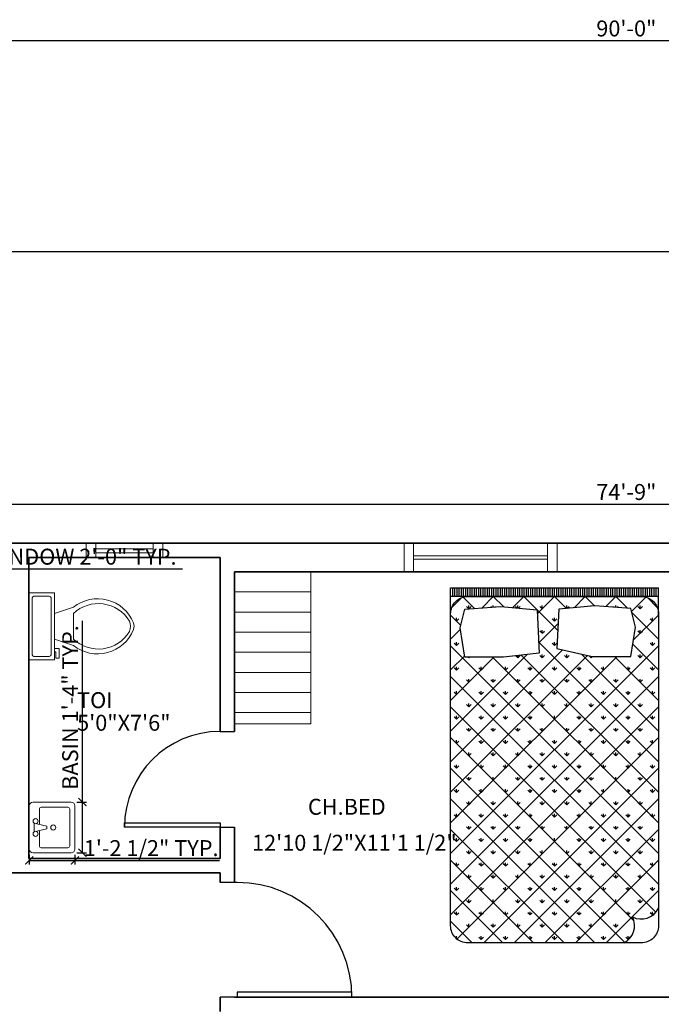
# Model space of a CAD drawing. Units: inches. Extents: x 3283068 to 3284536, y 3240756 to 3241803.
# Tile 15 of 19: x 3283598 to 3283799, y 3241494 to 3241803. Entities that reach past the tile are written whole.
import ezdxf

# ---------------------------------------------------------------- set-up
doc = ezdxf.new("R2010")
doc.units = ezdxf.units.IN
for name, color, linetype, lineweight in [('A-ANNO-DIMS', 2, 'Continuous', 18), ('A-AREA-IDEN', 7, 'Continuous', 18), ('A-FLOR-FIXT', 9, 'Continuous', 18), ('C-PROP', 7, 'Continuous', 25), ('door', 140, 'Continuous', 25), ('furniture', 40, 'Continuous', 18), ('wall', 20, 'Continuous', 35), ('wardrobe', 180, 'Continuous', 18), ('window', 100, 'Continuous', 18)]:
    doc.layers.add(name, color=color, linetype=linetype, lineweight=lineweight)
doc.layers.add('NOI THAT', color=42, linetype='Continuous')
doc.styles.get("Standard").update_dxf_attribs({"font": 'arial.ttf'})
doc.dimstyles.new('ISO-25', dxfattribs={"dimtxt": 5, "dimasz": 2.5, "dimexe": 1.25, "dimexo": 0.625, "dimtad": 1, "dimlunit": 4, "dimtxsty": 'Standard', "dimblk": 'ARCHTICK', "dimcen": 2.5, "dimadec": 0, "dimazin": 0, "dimtfac": 1, "dimtmove": 0, "dimatfit": 3, "dimfxl": 1, "dimarcsym": 0})

# ---------------------------------------------------------------- blocks, each defined once
blk = doc.blocks.new('*U6')
for p, q in [((0, 0), (0, -6)), ((-40, 0), (-40, -6))]:
    blk.add_line(p, q)
blk.add_lwpolyline([(0, 0), (0, 40), (-1.75, 40), (-1.75, 0)], close=True)
blk.add_arc((0, 0), 40, 90, 180)
blk = doc.blocks.new('*U5')
for p, q in [((-40, 0), (-40, 6)), ((0, 0), (0, 6))]:
    blk.add_line(p, q)
blk.add_lwpolyline([(0, 0), (0, -40), (-1.75, -40), (-1.75, 0)], close=True)
blk.add_arc((0, 0), 40, 180, 270)
blk = doc.blocks.new('*X15')
at = {"color": 0}
for p, q in [((-424.3, 0), (-424.3, 0)), ((-424.3, 0), (-424.3, 0)), ((-141.4, 0), (-141.4, 0)), ((-495, -70.6), (-495, -52)), ((-353.6, -60.2), (-353.6, -52)), ((-282.8, 0), (-282.8, 0)), ((-282.8, 0), (-282.8, 0)), ((-212.1, -65.8), (-212.1, -52)), ((-70.7, -70.7), (-70.7, -52)), ((70.7, -68.1), (70.7, -52)), ((212.1, -55), (212.1, -52)), ((282.8, 0), (282.8, 0)), ((353.6, -61.9), (353.6, -52)), ((424.3, 0), (424.3, 0)), ((495, -70.7), (495, -52)), ((-495.1, -70.6), (-508.2, -57.5)), ((-494.9, -70.6), (-481.7, -57.5)), ((-363.4, -60.9), (-366.8, -57.5)), ((-342.2, -59.3), (-340.3, -57.5)), ((-217.5, -65.3), (-225.4, -57.5)), ((-207.7, -66.2), (-198.9, -57.5)), ((-70.7, -70.7), (-84, -57.5)), ((-70.7, -70.7), (-57.5, -57.5)), ((68.3, -68.3), (57.5, -57.5)), ((73.6, -67.8), (84, -57.5)), ((344.1, -61.2), (340.3, -57.5)), ((361.7, -62.5), (366.8, -57.5)), ((495, -70.7), (481.7, -57.5)), ((495, -70.7), (508.2, -57.5)), ((-565.7, -141.4), (-578.9, -128.2)), ((-565.7, -141.4), (-565.7, -122.7)), ((-565.7, -141.4), (-552.4, -128.2)), ((0, -141.4), (-13.3, -128.2)), ((0, -141.4), (0, -122.7)), ((0, -141.4), (13.3, -128.2)), ((565.7, -141.4), (552.4, -128.2)), ((565.7, -141.4), (565.7, -122.7)), ((565.7, -141.4), (578.9, -128.2)), ((-70.7, -212.1), (-84, -198.9)), ((-70.7, -212.1), (-70.7, -193.4)), ((-70.7, -212.1), (-57.5, -198.9)), ((495, -212.1), (481.7, -198.9)), ((495, -212.1), (495, -193.4)), ((495, -212.1), (508.2, -198.9)), ((-565.7, -282.8), (-578.9, -269.6)), ((-565.7, -282.8), (-565.7, -264.1)), ((-565.7, -282.8), (-552.4, -269.6)), ((0, -282.8), (-13.3, -269.6)), ((0, -282.8), (0, -264.1)), ((0, -282.8), (13.3, -269.6)), ((565.7, -282.8), (552.4, -269.6)), ((565.7, -282.8), (565.7, -264.1)), ((565.7, -282.8), (578.9, -269.6)), ((-212.1, -353.6), (-212.1, -340.3)), ((-212.1, -353.6), (-198.9, -340.3)), ((-70.7, -353.6), (-84, -340.3)), ((-70.7, -353.6), (-70.7, -334.8)), ((-70.7, -353.6), (-57.5, -340.3)), ((70.7, -353.6), (57.5, -340.3)), ((70.7, -353.6), (70.7, -334.8)), ((70.7, -353.6), (84, -340.3)), ((495, -353.6), (481.7, -340.3)), ((495, -353.6), (495, -334.8)), ((495, -353.6), (508.2, -340.3)), ((-495, -353.6), (-499, -349.5)), ((-495, -353.6), (-495, -349.5)), ((-495, -353.6), (-491, -349.5)), ((-353.6, -353.6), (-357.6, -349.5)), ((-353.6, -353.6), (-353.6, -349.5)), ((-353.6, -353.6), (-349.5, -349.5)), ((-212.1, -353.6), (-224, -341.7)), ((212.1, -353.6), (200.4, -341.8)), ((212.1, -353.6), (212.1, -344.4)), ((212.1, -353.6), (220, -345.7)), ((353.6, -353.6), (345.7, -345.7)), ((353.6, -353.6), (353.6, -345.7)), ((353.6, -353.6), (361.4, -345.7)), ((-565.7, -424.3), (-578.9, -411)), ((-565.7, -424.3), (-565.7, -405.5)), ((-565.7, -424.3), (-552.4, -411)), ((-424.3, -424.3), (-437.5, -411)), ((-424.3, -424.3), (-424.3, -405.5)), ((-424.3, -424.3), (-411, -411)), ((-282.8, -424.3), (-296.1, -411)), ((-282.8, -424.3), (-282.8, -405.5)), ((-282.8, -424.3), (-269.6, -411)), ((-141.4, -424.3), (-154.7, -411)), ((-141.4, -424.3), (-141.4, -405.5)), ((-141.4, -424.3), (-128.2, -411)), ((0, -424.3), (-13.3, -411)), ((0, -424.3), (0, -405.5)), ((0, -424.3), (13.3, -411)), ((141.4, -424.3), (128.2, -411)), ((141.4, -424.3), (141.4, -405.5)), ((141.4, -424.3), (154.7, -411)), ((282.8, -424.3), (269.6, -411)), ((282.8, -424.3), (282.8, -405.5)), ((282.8, -424.3), (296.1, -411)), ((424.3, -424.3), (411, -411)), ((424.3, -424.3), (424.3, -405.5)), ((424.3, -424.3), (437.5, -411)), ((565.7, -424.3), (552.4, -411)), ((565.7, -424.3), (565.7, -405.5)), ((565.7, -424.3), (578.9, -411)), ((-495, -495), (-508.2, -481.7)), ((-495, -495), (-495, -476.2)), ((-495, -495), (-481.7, -481.7)), ((-353.6, -495), (-366.8, -481.7)), ((-353.6, -495), (-353.6, -476.2)), ((-353.6, -495), (-340.3, -481.7)), ((-212.1, -495), (-225.4, -481.7)), ((-212.1, -495), (-212.1, -476.2)), ((-212.1, -495), (-198.9, -481.7)), ((-70.7, -495), (-84, -481.7)), ((-70.7, -495), (-70.7, -476.2)), ((-70.7, -495), (-57.5, -481.7)), ((70.7, -495), (57.5, -481.7)), ((70.7, -495), (70.7, -476.2)), ((70.7, -495), (84, -481.7)), ((212.1, -495), (198.9, -481.7)), ((212.1, -495), (212.1, -476.2)), ((212.1, -495), (225.4, -481.7)), ((353.6, -495), (340.3, -481.7)), ((353.6, -495), (353.6, -476.2)), ((353.6, -495), (366.8, -481.7)), ((495, -495), (481.7, -481.7)), ((495, -495), (495, -476.2)), ((495, -495), (508.2, -481.7)), ((-565.7, -565.7), (-578.9, -552.4)), ((-565.7, -565.7), (-565.7, -546.9)), ((-565.7, -565.7), (-552.4, -552.4)), ((-424.3, -565.7), (-437.5, -552.4)), ((-424.3, -565.7), (-424.3, -546.9)), ((-424.3, -565.7), (-411, -552.4)), ((-282.8, -565.7), (-296.1, -552.4)), ((-282.8, -565.7), (-282.8, -546.9)), ((-282.8, -565.7), (-269.6, -552.4)), ((-141.4, -565.7), (-154.7, -552.4)), ((-141.4, -565.7), (-141.4, -546.9)), ((-141.4, -565.7), (-128.2, -552.4)), ((0, -565.7), (-13.3, -552.4)), ((0, -565.7), (0, -546.9)), ((0, -565.7), (13.3, -552.4)), ((141.4, -565.7), (128.2, -552.4)), ((141.4, -565.7), (141.4, -546.9)), ((141.4, -565.7), (154.7, -552.4)), ((282.8, -565.7), (269.6, -552.4)), ((282.8, -565.7), (282.8, -546.9)), ((282.8, -565.7), (296.1, -552.4)), ((424.3, -565.7), (411, -552.4)), ((424.3, -565.7), (424.3, -546.9)), ((424.3, -565.7), (437.5, -552.4)), ((565.7, -565.7), (552.4, -552.4)), ((565.7, -565.7), (565.7, -546.9)), ((565.7, -565.7), (578.9, -552.4)), ((-495, -636.4), (-508.2, -623.1)), ((-495, -636.4), (-495, -617.6)), ((-495, -636.4), (-481.7, -623.1)), ((-353.6, -636.4), (-366.8, -623.1)), ((-353.6, -636.4), (-353.6, -617.6)), ((-353.6, -636.4), (-340.3, -623.1)), ((-212.1, -636.4), (-225.4, -623.1)), ((-212.1, -636.4), (-212.1, -617.6)), ((-212.1, -636.4), (-198.9, -623.1)), ((-70.7, -636.4), (-84, -623.1)), ((-70.7, -636.4), (-70.7, -617.6)), ((-70.7, -636.4), (-57.5, -623.1)), ((70.7, -636.4), (57.5, -623.1)), ((70.7, -636.4), (70.7, -617.6)), ((70.7, -636.4), (84, -623.1)), ((212.1, -636.4), (198.9, -623.1)), ((212.1, -636.4), (212.1, -617.6)), ((212.1, -636.4), (225.4, -623.1)), ((353.6, -636.4), (340.3, -623.1)), ((353.6, -636.4), (353.6, -617.6)), ((353.6, -636.4), (366.8, -623.1)), ((495, -636.4), (481.7, -623.1)), ((495, -636.4), (495, -617.6)), ((495, -636.4), (508.2, -623.1)), ((-565.7, -707.1), (-578.9, -693.8)), ((-565.7, -707.1), (-565.7, -688.4)), ((-565.7, -707.1), (-552.4, -693.8)), ((-424.3, -707.1), (-437.5, -693.8)), ((-424.3, -707.1), (-424.3, -688.4)), ((-424.3, -707.1), (-411, -693.8)), ((-282.8, -707.1), (-296.1, -693.8)), ((-282.8, -707.1), (-282.8, -688.4)), ((-282.8, -707.1), (-269.6, -693.8)), ((-141.4, -707.1), (-154.7, -693.8)), ((-141.4, -707.1), (-141.4, -688.4)), ((-141.4, -707.1), (-128.2, -693.8)), ((0, -707.1), (-13.3, -693.8)), ((0, -707.1), (0, -688.4)), ((0, -707.1), (13.3, -693.8)), ((141.4, -707.1), (128.2, -693.8)), ((141.4, -707.1), (141.4, -688.4)), ((141.4, -707.1), (154.7, -693.8)), ((282.8, -707.1), (269.6, -693.8)), ((282.8, -707.1), (282.8, -688.4)), ((282.8, -707.1), (296.1, -693.8)), ((424.3, -707.1), (411, -693.8)), ((424.3, -707.1), (424.3, -688.4)), ((424.3, -707.1), (437.5, -693.8)), ((565.7, -707.1), (552.4, -693.8)), ((565.7, -707.1), (565.7, -688.4)), ((565.7, -707.1), (578.9, -693.8)), ((-495, -777.8), (-508.2, -764.6)), ((-495, -777.8), (-495, -759.1)), ((-495, -777.8), (-481.7, -764.6)), ((-353.6, -777.8), (-366.8, -764.6)), ((-353.6, -777.8), (-353.6, -759.1)), ((-353.6, -777.8), (-340.3, -764.6)), ((-212.1, -777.8), (-225.4, -764.6)), ((-212.1, -777.8), (-212.1, -759.1)), ((-212.1, -777.8), (-198.9, -764.6)), ((-70.7, -777.8), (-84, -764.6)), ((-70.7, -777.8), (-70.7, -759.1)), ((-70.7, -777.8), (-57.5, -764.6)), ((70.7, -777.8), (57.5, -764.6)), ((70.7, -777.8), (70.7, -759.1)), ((70.7, -777.8), (84, -764.6)), ((212.1, -777.8), (198.9, -764.6)), ((212.1, -777.8), (212.1, -759.1)), ((212.1, -777.8), (225.4, -764.6)), ((353.6, -777.8), (340.3, -764.6)), ((353.6, -777.8), (353.6, -759.1)), ((353.6, -777.8), (366.8, -764.6)), ((495, -777.8), (481.7, -764.6)), ((495, -777.8), (495, -759.1)), ((495, -777.8), (508.2, -764.6)), ((-565.7, -848.5), (-578.9, -835.3)), ((-565.7, -848.5), (-565.7, -829.8)), ((-565.7, -848.5), (-552.4, -835.3)), ((-424.3, -848.5), (-437.5, -835.3)), ((-424.3, -848.5), (-424.3, -829.8)), ((-424.3, -848.5), (-411, -835.3)), ((-282.8, -848.5), (-296.1, -835.3)), ((-282.8, -848.5), (-282.8, -829.8)), ((-282.8, -848.5), (-269.6, -835.3)), ((-141.4, -848.5), (-154.7, -835.3)), ((-141.4, -848.5), (-141.4, -829.8)), ((-141.4, -848.5), (-128.2, -835.3)), ((0, -848.5), (-13.3, -835.3)), ((0, -848.5), (0, -829.8)), ((0, -848.5), (13.3, -835.3)), ((141.4, -848.5), (128.2, -835.3)), ((141.4, -848.5), (141.4, -829.8)), ((141.4, -848.5), (154.7, -835.3)), ((282.8, -848.5), (269.6, -835.3)), ((282.8, -848.5), (282.8, -829.8)), ((282.8, -848.5), (296.1, -835.3)), ((424.3, -848.5), (411, -835.3)), ((424.3, -848.5), (424.3, -829.8)), ((424.3, -848.5), (437.5, -835.3)), ((565.7, -848.5), (552.4, -835.3)), ((565.7, -848.5), (565.7, -829.8)), ((565.7, -848.5), (578.9, -835.3)), ((-495, -919.2), (-508.2, -906)), ((-495, -919.2), (-495, -900.5)), ((-495, -919.2), (-481.7, -906)), ((-353.6, -919.2), (-366.8, -906)), ((-353.6, -919.2), (-353.6, -900.5)), ((-353.6, -919.2), (-340.3, -906)), ((-212.1, -919.2), (-225.4, -906)), ((-212.1, -919.2), (-212.1, -900.5)), ((-212.1, -919.2), (-198.9, -906)), ((-70.7, -919.2), (-84, -906)), ((-70.7, -919.2), (-70.7, -900.5)), ((-70.7, -919.2), (-57.5, -906)), ((70.7, -919.2), (57.5, -906)), ((70.7, -919.2), (70.7, -900.5)), ((70.7, -919.2), (84, -906)), ((212.1, -919.2), (198.9, -906)), ((212.1, -919.2), (212.1, -900.5)), ((212.1, -919.2), (225.4, -906)), ((353.6, -919.2), (340.3, -906)), ((353.6, -919.2), (353.6, -900.5)), ((353.6, -919.2), (366.8, -906)), ((495, -919.2), (481.7, -906)), ((495, -919.2), (495, -900.5)), ((495, -919.2), (508.2, -906)), ((-565.7, -989.9), (-578.9, -976.7)), ((-565.7, -989.9), (-565.7, -971.2)), ((-565.7, -989.9), (-552.4, -976.7)), ((-424.3, -989.9), (-437.5, -976.7)), ((-424.3, -989.9), (-424.3, -971.2)), ((-424.3, -989.9), (-411, -976.7)), ((-282.8, -989.9), (-296.1, -976.7)), ((-282.8, -989.9), (-282.8, -971.2)), ((-282.8, -989.9), (-269.6, -976.7)), ((-141.4, -989.9), (-154.7, -976.7)), ((-141.4, -989.9), (-141.4, -971.2)), ((-141.4, -989.9), (-128.2, -976.7)), ((0, -989.9), (-13.3, -976.7)), ((0, -989.9), (0, -971.2)), ((0, -989.9), (13.3, -976.7)), ((141.4, -989.9), (128.2, -976.7)), ((141.4, -989.9), (141.4, -971.2)), ((141.4, -989.9), (154.7, -976.7)), ((282.8, -989.9), (269.6, -976.7)), ((282.8, -989.9), (282.8, -971.2)), ((282.8, -989.9), (296.1, -976.7)), ((424.3, -989.9), (411, -976.7)), ((424.3, -989.9), (424.3, -971.2)), ((424.3, -989.9), (437.5, -976.7)), ((565.7, -989.9), (552.4, -976.7)), ((565.7, -989.9), (565.7, -971.2)), ((565.7, -989.9), (578.9, -976.7)), ((-495, -1060.7), (-508.2, -1047.4)), ((-495, -1060.7), (-495, -1041.9)), ((-495, -1060.7), (-481.7, -1047.4)), ((-353.6, -1060.7), (-366.8, -1047.4)), ((-353.6, -1060.7), (-353.6, -1041.9)), ((-353.6, -1060.7), (-340.3, -1047.4)), ((-212.1, -1060.7), (-225.4, -1047.4)), ((-212.1, -1060.7), (-212.1, -1041.9)), ((-212.1, -1060.7), (-198.9, -1047.4)), ((-70.7, -1060.7), (-84, -1047.4)), ((-70.7, -1060.7), (-70.7, -1041.9)), ((-70.7, -1060.7), (-57.5, -1047.4)), ((70.7, -1060.7), (57.5, -1047.4)), ((70.7, -1060.7), (70.7, -1041.9)), ((70.7, -1060.7), (84, -1047.4)), ((212.1, -1060.7), (198.9, -1047.4)), ((212.1, -1060.7), (212.1, -1041.9)), ((212.1, -1060.7), (225.4, -1047.4)), ((353.6, -1060.7), (340.3, -1047.4)), ((353.6, -1060.7), (353.6, -1041.9)), ((353.6, -1060.7), (366.8, -1047.4)), ((495, -1060.7), (481.7, -1047.4)), ((495, -1060.7), (495, -1041.9)), ((495, -1060.7), (508.2, -1047.4)), ((-565.7, -1131.4), (-578.9, -1118.1)), ((-565.7, -1131.4), (-565.7, -1112.6)), ((-565.7, -1131.4), (-552.4, -1118.1)), ((-424.3, -1131.4), (-437.5, -1118.1)), ((-424.3, -1131.4), (-424.3, -1112.6)), ((-424.3, -1131.4), (-411, -1118.1)), ((-282.8, -1131.4), (-296.1, -1118.1)), ((-282.8, -1131.4), (-282.8, -1112.6)), ((-282.8, -1131.4), (-269.6, -1118.1)), ((-141.4, -1131.4), (-154.7, -1118.1)), ((-141.4, -1131.4), (-141.4, -1112.6)), ((-141.4, -1131.4), (-128.2, -1118.1)), ((0, -1131.4), (-13.3, -1118.1)), ((0, -1131.4), (0, -1112.6)), ((0, -1131.4), (13.3, -1118.1)), ((141.4, -1131.4), (128.2, -1118.1)), ((141.4, -1131.4), (141.4, -1112.6)), ((141.4, -1131.4), (154.7, -1118.1)), ((282.8, -1131.4), (269.6, -1118.1)), ((282.8, -1131.4), (282.8, -1112.6)), ((282.8, -1131.4), (296.1, -1118.1)), ((424.3, -1131.4), (411, -1118.1)), ((424.3, -1131.4), (424.3, -1112.6)), ((424.3, -1131.4), (437.5, -1118.1)), ((565.7, -1131.4), (552.4, -1118.1)), ((565.7, -1131.4), (565.7, -1112.6)), ((565.7, -1131.4), (578.9, -1118.1)), ((-495, -1202.1), (-508.2, -1188.8)), ((-495, -1202.1), (-495, -1183.3)), ((-495, -1202.1), (-481.7, -1188.8)), ((-353.6, -1202.1), (-366.8, -1188.8)), ((-353.6, -1202.1), (-353.6, -1183.3)), ((-353.6, -1202.1), (-340.3, -1188.8)), ((-212.1, -1202.1), (-225.4, -1188.8)), ((-212.1, -1202.1), (-212.1, -1183.3)), ((-212.1, -1202.1), (-198.9, -1188.8)), ((-70.7, -1202.1), (-84, -1188.8)), ((-70.7, -1202.1), (-70.7, -1183.3)), ((-70.7, -1202.1), (-57.5, -1188.8)), ((70.7, -1202.1), (57.5, -1188.8)), ((70.7, -1202.1), (70.7, -1183.3)), ((70.7, -1202.1), (84, -1188.8)), ((212.1, -1202.1), (198.9, -1188.8)), ((212.1, -1202.1), (212.1, -1183.3)), ((212.1, -1202.1), (225.4, -1188.8)), ((353.6, -1202.1), (340.3, -1188.8)), ((353.6, -1202.1), (353.6, -1183.3)), ((353.6, -1202.1), (366.8, -1188.8)), ((495, -1202.1), (481.7, -1188.8)), ((495, -1202.1), (495, -1183.3)), ((495, -1202.1), (508.2, -1188.8)), ((-565.7, -1272.8), (-578.9, -1259.5)), ((-565.7, -1272.8), (-565.7, -1254)), ((-565.7, -1272.8), (-552.4, -1259.5)), ((-424.3, -1272.8), (-437.5, -1259.5)), ((-424.3, -1272.8), (-424.3, -1254)), ((-424.3, -1272.8), (-411, -1259.5)), ((-282.8, -1272.8), (-296.1, -1259.5)), ((-282.8, -1272.8), (-282.8, -1254)), ((-282.8, -1272.8), (-269.6, -1259.5)), ((-141.4, -1272.8), (-154.7, -1259.5)), ((-141.4, -1272.8), (-141.4, -1254)), ((-141.4, -1272.8), (-128.2, -1259.5)), ((0, -1272.8), (-13.3, -1259.5)), ((0, -1272.8), (0, -1254)), ((0, -1272.8), (13.3, -1259.5)), ((141.4, -1272.8), (128.2, -1259.5)), ((141.4, -1272.8), (141.4, -1254)), ((141.4, -1272.8), (154.7, -1259.5)), ((282.8, -1272.8), (269.6, -1259.5)), ((282.8, -1272.8), (282.8, -1254)), ((282.8, -1272.8), (296.1, -1259.5)), ((424.3, -1272.8), (411, -1259.5)), ((424.3, -1272.8), (424.3, -1254)), ((424.3, -1272.8), (437.5, -1259.5)), ((565.7, -1272.8), (552.4, -1259.5)), ((565.7, -1272.8), (565.7, -1254)), ((565.7, -1272.8), (578.9, -1259.5)), ((-495, -1343.5), (-508.2, -1330.2)), ((-495, -1343.5), (-495, -1324.8)), ((-495, -1343.5), (-481.7, -1330.2)), ((-353.6, -1343.5), (-366.8, -1330.2)), ((-353.6, -1343.5), (-353.6, -1324.8)), ((-353.6, -1343.5), (-340.3, -1330.2)), ((-212.1, -1343.5), (-225.4, -1330.2)), ((-212.1, -1343.5), (-212.1, -1324.8)), ((-212.1, -1343.5), (-198.9, -1330.2)), ((-70.7, -1343.5), (-84, -1330.2)), ((-70.7, -1343.5), (-70.7, -1324.8)), ((-70.7, -1343.5), (-57.5, -1330.2)), ((70.7, -1343.5), (57.5, -1330.2)), ((70.7, -1343.5), (70.7, -1324.8)), ((70.7, -1343.5), (84, -1330.2)), ((212.1, -1343.5), (198.9, -1330.2)), ((212.1, -1343.5), (212.1, -1324.8)), ((212.1, -1343.5), (225.4, -1330.2)), ((353.6, -1343.5), (340.3, -1330.2)), ((353.6, -1343.5), (353.6, -1324.8)), ((353.6, -1343.5), (366.8, -1330.2)), ((495, -1343.5), (481.7, -1330.2)), ((495, -1343.5), (495, -1324.8)), ((495, -1343.5), (508.2, -1330.2)), ((-565.7, -1414.2), (-578.9, -1401)), ((-565.7, -1414.2), (-565.7, -1395.5)), ((-565.7, -1414.2), (-552.4, -1401)), ((-424.3, -1414.2), (-437.5, -1401)), ((-424.3, -1414.2), (-424.3, -1395.5)), ((-424.3, -1414.2), (-411, -1401)), ((-282.8, -1414.2), (-296.1, -1401)), ((-282.8, -1414.2), (-282.8, -1395.5)), ((-282.8, -1414.2), (-269.6, -1401)), ((-141.4, -1414.2), (-154.7, -1401)), ((-141.4, -1414.2), (-141.4, -1395.5)), ((-141.4, -1414.2), (-128.2, -1401)), ((0, -1414.2), (-13.3, -1401)), ((0, -1414.2), (0, -1395.5)), ((0, -1414.2), (13.3, -1401)), ((141.4, -1414.2), (128.2, -1401)), ((141.4, -1414.2), (141.4, -1395.5)), ((141.4, -1414.2), (154.7, -1401)), ((282.8, -1414.2), (269.6, -1401)), ((282.8, -1414.2), (282.8, -1395.5)), ((282.8, -1414.2), (296.1, -1401)), ((424.3, -1414.2), (411, -1401)), ((424.3, -1414.2), (424.3, -1395.5)), ((424.3, -1414.2), (437.5, -1401)), ((565.7, -1414.2), (552.4, -1401)), ((565.7, -1414.2), (565.7, -1395.5)), ((565.7, -1414.2), (578.9, -1401)), ((-495, -1484.9), (-508.2, -1471.7)), ((-495, -1484.9), (-495, -1466.2)), ((-495, -1484.9), (-481.7, -1471.7)), ((-353.6, -1484.9), (-366.8, -1471.7)), ((-353.6, -1484.9), (-353.6, -1466.2)), ((-353.6, -1484.9), (-340.3, -1471.7)), ((-212.1, -1484.9), (-225.4, -1471.7)), ((-212.1, -1484.9), (-212.1, -1466.2)), ((-212.1, -1484.9), (-198.9, -1471.7)), ((-70.7, -1484.9), (-84, -1471.7)), ((-70.7, -1484.9), (-70.7, -1466.2)), ((-70.7, -1484.9), (-57.5, -1471.7)), ((70.7, -1484.9), (57.5, -1471.7)), ((70.7, -1484.9), (70.7, -1466.2)), ((70.7, -1484.9), (84, -1471.7)), ((212.1, -1484.9), (198.9, -1471.7)), ((212.1, -1484.9), (212.1, -1466.2)), ((212.1, -1484.9), (225.4, -1471.7)), ((353.6, -1484.9), (340.3, -1471.7)), ((353.6, -1484.9), (353.6, -1466.2)), ((353.6, -1484.9), (366.8, -1471.7)), ((495, -1484.9), (481.7, -1471.7)), ((495, -1484.9), (495, -1466.2)), ((495, -1484.9), (508.2, -1471.7)), ((-565.7, -1555.6), (-578.9, -1542.4)), ((-565.7, -1555.6), (-565.7, -1536.9)), ((-565.7, -1555.6), (-552.4, -1542.4)), ((-424.3, -1555.6), (-437.5, -1542.4)), ((-424.3, -1555.6), (-424.3, -1536.9)), ((-424.3, -1555.6), (-411, -1542.4)), ((-282.8, -1555.6), (-296.1, -1542.4)), ((-282.8, -1555.6), (-282.8, -1536.9)), ((-282.8, -1555.6), (-269.6, -1542.4)), ((-141.4, -1555.6), (-154.7, -1542.4)), ((-141.4, -1555.6), (-141.4, -1536.9)), ((-141.4, -1555.6), (-128.2, -1542.4)), ((0, -1555.6), (-13.3, -1542.4)), ((0, -1555.6), (0, -1536.9)), ((0, -1555.6), (13.3, -1542.4)), ((141.4, -1555.6), (128.2, -1542.4)), ((141.4, -1555.6), (141.4, -1536.9)), ((141.4, -1555.6), (154.7, -1542.4)), ((282.8, -1555.6), (269.6, -1542.4)), ((282.8, -1555.6), (282.8, -1536.9)), ((282.8, -1555.6), (296.1, -1542.4)), ((424.3, -1555.6), (411, -1542.4)), ((424.3, -1555.6), (424.3, -1536.9)), ((424.3, -1555.6), (437.5, -1542.4)), ((565.7, -1555.6), (552.4, -1542.4)), ((565.7, -1555.6), (565.7, -1536.9)), ((565.7, -1555.6), (578.9, -1542.4)), ((-495, -1626.3), (-508.2, -1613.1)), ((-495, -1626.3), (-495, -1607.6)), ((-495, -1626.3), (-481.7, -1613.1)), ((-353.6, -1626.3), (-366.8, -1613.1)), ((-353.6, -1626.3), (-353.6, -1607.6)), ((-353.6, -1626.3), (-340.3, -1613.1)), ((-212.1, -1626.3), (-225.4, -1613.1)), ((-212.1, -1626.3), (-212.1, -1607.6)), ((-212.1, -1626.3), (-198.9, -1613.1)), ((-70.7, -1626.3), (-84, -1613.1)), ((-70.7, -1626.3), (-70.7, -1607.6)), ((-70.7, -1626.3), (-57.5, -1613.1)), ((70.7, -1626.3), (57.5, -1613.1)), ((70.7, -1626.3), (70.7, -1607.6)), ((70.7, -1626.3), (84, -1613.1)), ((212.1, -1626.3), (198.9, -1613.1)), ((212.1, -1626.3), (212.1, -1607.6)), ((212.1, -1626.3), (225.4, -1613.1)), ((353.6, -1626.3), (340.3, -1613.1)), ((353.6, -1626.3), (353.6, -1607.6)), ((353.6, -1626.3), (366.8, -1613.1)), ((495, -1626.3), (481.7, -1613.1)), ((495, -1626.3), (495, -1607.6)), ((495, -1626.3), (508.2, -1613.1)), ((-565.7, -1697.1), (-578.9, -1683.8)), ((-565.7, -1697.1), (-565.7, -1678.3)), ((-565.7, -1697.1), (-552.4, -1683.8)), ((-424.3, -1697.1), (-437.5, -1683.8)), ((-424.3, -1697.1), (-424.3, -1678.3)), ((-424.3, -1697.1), (-411, -1683.8)), ((-282.8, -1697.1), (-296.1, -1683.8)), ((-282.8, -1697.1), (-282.8, -1678.3)), ((-282.8, -1697.1), (-269.6, -1683.8)), ((-141.4, -1697.1), (-154.7, -1683.8)), ((-141.4, -1697.1), (-141.4, -1678.3)), ((-141.4, -1697.1), (-128.2, -1683.8)), ((0, -1697.1), (-13.3, -1683.8)), ((0, -1697.1), (0, -1678.3)), ((0, -1697.1), (13.3, -1683.8)), ((141.4, -1697.1), (128.2, -1683.8)), ((141.4, -1697.1), (141.4, -1678.3)), ((141.4, -1697.1), (154.7, -1683.8)), ((282.8, -1697.1), (269.6, -1683.8)), ((282.8, -1697.1), (282.8, -1678.3)), ((282.8, -1697.1), (296.1, -1683.8)), ((424.3, -1697.1), (411, -1683.8)), ((424.3, -1697.1), (424.3, -1678.3)), ((424.3, -1697.1), (437.5, -1683.8)), ((565.7, -1697.1), (552.4, -1683.8)), ((565.7, -1697.1), (565.7, -1678.3)), ((565.7, -1697.1), (578.9, -1683.8)), ((-495, -1767.8), (-508.2, -1754.5)), ((-495, -1767.8), (-495, -1749)), ((-495, -1767.8), (-481.7, -1754.5)), ((-353.6, -1767.8), (-366.8, -1754.5)), ((-353.6, -1767.8), (-353.6, -1749)), ((-353.6, -1767.8), (-340.3, -1754.5)), ((-212.1, -1767.8), (-225.4, -1754.5)), ((-212.1, -1767.8), (-212.1, -1749)), ((-212.1, -1767.8), (-198.9, -1754.5)), ((-70.7, -1767.8), (-84, -1754.5)), ((-70.7, -1767.8), (-70.7, -1749)), ((-70.7, -1767.8), (-57.5, -1754.5)), ((70.7, -1767.8), (57.5, -1754.5)), ((70.7, -1767.8), (70.7, -1749)), ((70.7, -1767.8), (84, -1754.5)), ((212.1, -1767.8), (198.9, -1754.5)), ((212.1, -1767.8), (212.1, -1749)), ((212.1, -1767.8), (225.4, -1754.5)), ((353.6, -1767.8), (340.3, -1754.5)), ((353.6, -1767.8), (353.6, -1749)), ((353.6, -1767.8), (366.8, -1754.5)), ((495, -1767.8), (481.7, -1754.5)), ((495, -1767.8), (495, -1749)), ((495, -1767.8), (508.2, -1754.5)), ((-565.7, -1838.5), (-578.9, -1825.2)), ((-565.7, -1838.5), (-565.7, -1819.7)), ((-565.7, -1838.5), (-552.4, -1825.2)), ((-424.3, -1838.5), (-437.5, -1825.2)), ((-424.3, -1838.5), (-424.3, -1819.7)), ((-424.3, -1838.5), (-411, -1825.2)), ((-282.8, -1838.5), (-296.1, -1825.2)), ((-282.8, -1838.5), (-282.8, -1819.7)), ((-282.8, -1838.5), (-269.6, -1825.2)), ((-141.4, -1838.5), (-154.7, -1825.2)), ((-141.4, -1838.5), (-141.4, -1819.7)), ((-141.4, -1838.5), (-128.2, -1825.2)), ((0, -1838.5), (-13.3, -1825.2)), ((0, -1838.5), (0, -1819.7)), ((0, -1838.5), (13.3, -1825.2)), ((141.4, -1838.5), (128.2, -1825.2)), ((141.4, -1838.5), (141.4, -1819.7)), ((141.4, -1838.5), (154.7, -1825.2)), ((282.8, -1838.5), (269.6, -1825.2)), ((282.8, -1838.5), (282.8, -1819.7)), ((282.8, -1838.5), (296.1, -1825.2)), ((424.3, -1838.5), (411, -1825.2)), ((424.3, -1838.5), (424.3, -1819.7)), ((424.3, -1838.5), (437.5, -1825.2)), ((565.7, -1838.5), (552.4, -1825.2)), ((565.7, -1838.5), (565.7, -1819.7)), ((565.7, -1838.5), (578.9, -1825.2)), ((-495, -1909.2), (-508.2, -1895.9)), ((-495, -1909.2), (-495, -1890.4)), ((-495, -1909.2), (-481.7, -1895.9)), ((-353.6, -1909.2), (-366.8, -1895.9)), ((-353.6, -1909.2), (-353.6, -1890.4)), ((-353.6, -1909.2), (-340.3, -1895.9)), ((-212.1, -1909.2), (-225.4, -1895.9)), ((-212.1, -1909.2), (-212.1, -1890.4)), ((-212.1, -1909.2), (-198.9, -1895.9)), ((-70.7, -1909.2), (-84, -1895.9)), ((-70.7, -1909.2), (-70.7, -1890.4)), ((-70.7, -1909.2), (-57.5, -1895.9)), ((70.7, -1909.2), (57.5, -1895.9)), ((70.7, -1909.2), (70.7, -1890.4)), ((70.7, -1909.2), (84, -1895.9)), ((212.1, -1909.2), (198.9, -1895.9)), ((212.1, -1909.2), (212.1, -1890.4)), ((212.1, -1909.2), (225.4, -1895.9)), ((353.6, -1909.2), (340.3, -1895.9)), ((353.6, -1909.2), (353.6, -1890.4)), ((353.6, -1909.2), (366.8, -1895.9)), ((-565.7, -1975.4), (-565.7, -1961.1)), ((-563.2, -1977.5), (-552.4, -1966.6)), ((-424.3, -1979.9), (-437.5, -1966.6)), ((-424.3, -1979.9), (-424.3, -1961.1)), ((-424.3, -1979.9), (-411, -1966.6)), ((-282.8, -1979.9), (-296.1, -1966.6)), ((-282.8, -1979.9), (-282.8, -1961.1)), ((-282.8, -1979.9), (-269.6, -1966.6)), ((-141.4, -1979.9), (-154.7, -1966.6)), ((-141.4, -1979.9), (-141.4, -1961.1)), ((-141.4, -1979.9), (-128.2, -1966.6)), ((0, -1979.9), (-13.3, -1966.6)), ((0, -1979.9), (0, -1961.1)), ((0, -1979.9), (13.3, -1966.6)), ((141.4, -1979.9), (128.2, -1966.6)), ((141.4, -1979.9), (141.4, -1961.1)), ((141.4, -1979.9), (154.7, -1966.6)), ((282.8, -1979.9), (269.6, -1966.6)), ((282.8, -1979.9), (282.8, -1961.1)), ((282.8, -1979.9), (296.1, -1966.6)), ((424.3, -1979.9), (411, -1966.6)), ((424.3, -1979.9), (424.3, -1961.1)), ((424.3, -1979.9), (437.5, -1966.6))]:
    blk.add_line(p, q, dxfattribs=at)
blk = doc.blocks.new('*X14')
at = {"color": 0}
for p, q in [((-592.6, -62.3), (-537.7, -7.4)), ((-462.1, -68.2), (-526.7, -3.6)), ((-418.5, -65), (-353.6, 0)), ((-295.4, -58.1), (-353.6, 0)), ((-240, -63.3), (-176.8, 0)), ((18.9, -195.7), (-176.8, 0)), ((-99.9, -99.9), (0, 0)), ((68.3, -68.3), (0, 0)), ((112.6, -64.2), (176.8, 0)), ((230.1, -53.3), (176.8, 0)), ((295.9, -57.6), (353.6, 0)), ((420.4, -66.9), (353.6, 0)), ((445.5, -84.9), (526.7, -3.6)), ((592.6, -62.3), (537.7, -7.4)), ((-540.7, -166.4), (-600, -107.1)), ((600, -246.4), (447.8, -94.3)), ((456.5, -250.6), (600, -107.1)), ((-92.1, -268.9), (21, -155.8)), ((-600, -246.4), (-542.7, -189.2)), ((-600, -1483.9), (600, -283.9)), ((600, -1483.9), (-600, -283.9)), ((600, -953.6), (-92.5, -261.1)), ((600, -423.2), (452.5, -275.7)), ((-600, -953.6), (46, -307.5)), ((-600, -776.8), (-157.3, -334.1)), ((-600, -1130.3), (190.7, -339.6)), ((600, -1130.3), (-192.3, -338.1)), ((600, -776.8), (154.9, -331.7)), ((-600, -423.2), (-518.4, -341.7)), ((-600, -1307.1), (361.4, -345.7)), ((-600, -600), (-349.5, -349.5)), ((600, -1307.1), (-357.6, -349.5)), ((600, -600), (345.7, -345.7)), ((-600, -1660.7), (600, -460.7)), ((600, -1660.7), (-600, -460.7)), ((-600, -1837.4), (600, -637.4)), ((585.1, -1822.5), (-600, -637.4)), ((458.4, -1872.6), (-600, -814.2)), ((-563.2, -1977.5), (600, -814.2)), ((405.9, -1996.8), (-600, -991)), ((-409, -2000), (600, -991)), ((232.2, -2000), (-600, -1167.8)), ((-232.2, -2000), (600, -1167.8)), ((55.5, -2000), (-600, -1344.5)), ((-55.5, -2000), (600, -1344.5)), ((-121.3, -2000), (-600, -1521.3)), ((121.3, -2000), (600, -1521.3)), ((-298.1, -2000), (-600, -1698.1)), ((298.1, -2000), (600, -1698.1)), ((-474.9, -2000), (-600, -1874.9))]:
    blk.add_line(p, q, dxfattribs=at)
blk = doc.blocks.new('*X16')
at = {"color": 0}
for p, q in [((-587.5, 0), (-587.5, 50)), ((-575, 0), (-575, 50)), ((-562.5, 0), (-562.5, 50)), ((-550, 0), (-550, 50)), ((-537.5, 0), (-537.5, 50)), ((-525, 0), (-525, 50)), ((-512.5, 0), (-512.5, 50)), ((-500, 0), (-500, 50)), ((-487.5, 0), (-487.5, 50)), ((-475, 0), (-475, 50)), ((-462.5, 0), (-462.5, 50)), ((-450, 0), (-450, 50)), ((-437.5, 0), (-437.5, 50)), ((-425, 0), (-425, 50)), ((-412.5, 0), (-412.5, 50)), ((-400, 0), (-400, 50)), ((-387.5, 0), (-387.5, 50)), ((-375, 0), (-375, 50)), ((-362.5, 0), (-362.5, 50)), ((-350, 0), (-350, 50)), ((-337.5, 0), (-337.5, 50)), ((-325, 0), (-325, 50)), ((-312.5, 0), (-312.5, 50)), ((-300, 0), (-300, 50)), ((-287.5, 0), (-287.5, 50)), ((-275, 0), (-275, 50)), ((-262.5, 0), (-262.5, 50)), ((-250, 0), (-250, 50)), ((-237.5, 0), (-237.5, 50)), ((-225, 0), (-225, 50)), ((-212.5, 0), (-212.5, 50)), ((-200, 0), (-200, 50)), ((-187.5, 0), (-187.5, 50)), ((-175, 0), (-175, 50)), ((-162.5, 0), (-162.5, 50)), ((-150, 0), (-150, 50)), ((-137.5, 0), (-137.5, 50)), ((-125, 0), (-125, 50)), ((-112.5, 0), (-112.5, 50)), ((-100, 0), (-100, 50)), ((-87.5, 0), (-87.5, 50)), ((-75, 0), (-75, 50)), ((-62.5, 0), (-62.5, 50)), ((-50, 0), (-50, 50)), ((-37.5, 0), (-37.5, 50)), ((-25, 0), (-25, 50)), ((-12.5, 0), (-12.5, 50)), ((0, 0), (0, 50)), ((12.5, 0), (12.5, 50)), ((25, 0), (25, 50)), ((37.5, 0), (37.5, 50)), ((50, 0), (50, 50)), ((62.5, 0), (62.5, 50)), ((75, 0), (75, 50)), ((87.5, 0), (87.5, 50)), ((100, 0), (100, 50)), ((112.5, 0), (112.5, 50)), ((125, 0), (125, 50)), ((137.5, 0), (137.5, 50)), ((150, 0), (150, 50)), ((162.5, 0), (162.5, 50)), ((175, 0), (175, 50)), ((187.5, 0), (187.5, 50)), ((200, 0), (200, 50)), ((212.5, 0), (212.5, 50)), ((225, 0), (225, 50)), ((237.5, 0), (237.5, 50)), ((250, 0), (250, 50)), ((262.5, 0), (262.5, 50)), ((275, 0), (275, 50)), ((287.5, 0), (287.5, 50)), ((300, 0), (300, 50)), ((312.5, 0), (312.5, 50)), ((325, 0), (325, 50)), ((337.5, 0), (337.5, 50)), ((350, 0), (350, 50)), ((362.5, 0), (362.5, 50)), ((375, 0), (375, 50)), ((387.5, 0), (387.5, 50)), ((400, 0), (400, 50)), ((412.5, 0), (412.5, 50)), ((425, 0), (425, 50)), ((437.5, 0), (437.5, 50)), ((450, 0), (450, 50)), ((462.5, 0), (462.5, 50)), ((475, 0), (475, 50)), ((487.5, 0), (487.5, 50)), ((500, 0), (500, 50)), ((512.5, 0), (512.5, 50)), ((525, 0), (525, 50)), ((537.5, 0), (537.5, 50)), ((550, 0), (550, 50)), ((562.5, 0), (562.5, 50)), ((575, 0), (575, 50)), ((587.5, 0), (587.5, 50))]:
    blk.add_line(p, q, dxfattribs=at)
blk = doc.blocks.new('A$C5BFD579E')
at = {"layer": 'NOI THAT'}
for p, q in [((0, 2050), (1200, 2050)), ((0, 1885.1), (0, 2050)), ((1200, 1885.1), (1200, 2050))]:
    blk.add_line(p, q, dxfattribs=at)
blk.add_lwpolyline([(100, 2000), (1100, 2000, -0.414214), (1200, 1900), (1200, 100, -0.414214), (1100, 0), (100, 0, -0.414214), (0, 100), (0, 1900, -0.414214)], format="xyb", close=True, dxfattribs=at)
blk.add_lwpolyline([(1200, 2000), (0, 2000)], dxfattribs=at)
for points in [[(290.9, 1943.1), (499, 1923.9), (510.6, 1673.6), (306.3, 1650.5), (82.8, 1650.5), (55.8, 1819.9), (82.8, 1927.7)], [(833.3, 1947), (625.2, 1927.7), (613.6, 1699.6), (817.9, 1654.3), (1041.4, 1654.3), (1068.3, 1823.8), (1041.4, 1931.6)]]:
    blk.add_lwpolyline(points, close=True, dxfattribs=at)
for centre, start, end in [((1100, 250), 243.4349, 333.4349), ((950, 100), 296.5651, 26.5651)]:
    blk.add_arc(centre, 111.8, start, end, dxfattribs=at)
for name in ['*X16', '*X14', '*X15']:
    blk.add_blockref(name, (600, 2000), dxfattribs=at)
blk = doc.blocks.new('*U22')
for p, q in [((241.3, -152.4), (241.3, -50.8)), ((-254, -215.9), (-203.2, -215.9)), ((-254, -241.3), (-254, -215.9)), ((-203.2, -215.9), (-203.2, -203.2)), ((-177.8, -203.2), (-177.8, -241.3)), ((-101.6, -203.2), (-152.4, -355.6)), ((101.6, -203.2), (152.4, -355.6)), ((-177.8, -241.3), (-254, -241.3)), ((101.6, -355.6), (-101.6, -355.6))]:
    blk.add_line(p, q)
blk.add_lwpolyline([(266.7, -203.2), (266.7, 0), (-266.7, 0), (-266.7, -203.2)], close=True)
for points in [[(-241.3, -50.8), (-241.3, -152.4)], [(215.9, -25.4), (-215.9, -25.4)], [(-215.9, -177.8), (215.9, -177.8)]]:
    blk.add_lwpolyline(points)
for centre, radius, start, end in [((-219.1, -47.6), 22.5, 81.8699, 188.1301), ((219.1, -47.6), 22.5, 351.8699, 98.1301), ((-219.1, -155.6), 22.5, 171.8699, 278.1301), ((219.1, -155.6), 22.5, 261.8699, 8.1301), ((89.4, -548.1), 309.1, 141.46911, 247.97143), ((106.7, -554.2), 287.8, 136.36773, 238.94682), ((-89.4, -548.1), 309.1, 292.02843, 38.53071), ((-106.7, -554.2), 287.8, 301.05301, 43.63209), ((0, -708.1), 101.6, 245.73182, 294.26817), ((0, -736.6), 101.6, 254.86053, 285.13947)]:
    blk.add_arc(centre, radius, start, end)
blk = doc.blocks.new('_ArchTick')
at = {"color": 0, "linetype": 'ByBlock', "const_width": 0.15}
blk.add_lwpolyline([(-0.5, -0.5), (0.5, 0.5)], dxfattribs=at)
blk = doc.blocks.new('*D25')
at = {"layer": 'A-ANNO-DIMS', "color": 0, "lineweight": -2, "transparency": 16777216}
for p, q in [((3283339.59, 3241639.73), (3283339.59, 3241652.58)), ((3283339.59, 3241651.33), (3284236.59, 3241651.33)), ((3284236.59, 3241639.73), (3284236.59, 3241652.58))]:
    blk.add_line(p, q, dxfattribs=at)
at = {"layer": 'Defpoints', "color": 0, "transparency": 16777216}
for p in [(3284236.59, 3241651.33), (3283339.59, 3241639.1), (3284236.59, 3241639.1)]:
    blk.add_point(p, dxfattribs=at)
at = {"layer": 'A-ANNO-DIMS', "color": 0, "lineweight": -2, "transparency": 16777216, "xscale": 2.5, "yscale": 2.5, "zscale": 2.5, "rotation": 180}
blk.add_blockref('_ArchTick', (3283339.59, 3241651.33), dxfattribs=at)
at = {"layer": 'A-ANNO-DIMS', "color": 0, "lineweight": -2, "transparency": 16777216, "xscale": 2.5, "yscale": 2.5, "zscale": 2.5}
blk.add_blockref('_ArchTick', (3284236.59, 3241651.33), dxfattribs=at)
at = {"layer": 'A-ANNO-DIMS', "color": 0, "transparency": 16777216, "insert": (3283788.09, 3241654.51), "char_height": 5, "attachment_point": 5}
blk.add_mtext('74\'-9"', dxfattribs=at)
blk = doc.blocks.new('WIN-48IN-9IN-WALL')
for p, q in [((0, 9), (48, 9)), ((0, 0), (0, 9)), ((3, 0), (3, 9)), ((45, 9), (45, 0)), ((48, 9), (48, 0)), ((3, 5), (45, 5)), ((3, 4), (45, 4)), ((48, 0), (0, 0))]:
    blk.add_line(p, q)
blk = doc.blocks.new('WIN-24IN-4_5IN-WALL')
for p, q in [((0, 4.5), (24, 4.5)), ((0, 0), (0, 4.5)), ((3, 0), (3, 4.5)), ((21, 4.5), (21, 0)), ((24, 4.5), (24, 0)), ((24, 0), (0, 0)), ((3, 2.73), (21, 2.73)), ((3, 1.44), (21, 1.44))]:
    blk.add_line(p, q)
blk = doc.blocks.new('LAVATORY-COMPACT')
for p, q in [((13.12, 15.9), (1.19, 15.9)), ((0, 14.71), (0, 1.19)), ((3.18, 8.94), (3.18, 13.71)), ((3.78, 14.31), (12.12, 14.31)), ((12.72, 13.71), (12.72, 2.19)), ((14.31, 1.19), (14.31, 14.71)), ((1.59, 6.76), (1.59, 9.14)), ((5.56, 8.35), (2.38, 9.14)), ((2.38, 6.76), (5.56, 7.55)), ((3.18, 2.19), (3.18, 6.96)), ((5.56, 7.55), (5.56, 8.35)), ((1.19, 0), (13.12, 0)), ((12.12, 1.59), (3.78, 1.59))]:
    blk.add_line(p, q)
for centre in [(1.99, 9.94), (1.99, 5.96), (7.55, 7.95)]:
    blk.add_circle(centre, 0.795)
for centre, radius, start, end in [((1.19, 14.71), 1.19, 90, 180), ((13.12, 14.71), 1.19, 0, 90), ((3.78, 13.71), 0.596, 90, 180), ((12.12, 13.71), 0.596, 0, 90), ((1.19, 1.19), 1.19, 180, 270), ((3.78, 2.19), 0.596, 180, 270), ((12.12, 2.19), 0.596, 270, 0), ((13.12, 1.19), 1.19, 270, 0)]:
    blk.add_arc(centre, radius, start, end)
blk = doc.blocks.new('*D43')
at = {"layer": 'A-ANNO-DIMS', "color": 0, "lineweight": -2, "transparency": 16777216}
for p, q in [((3283557.81, 3241633.98), (3283557.81, 3241629.75)), ((3283581.81, 3241633.98), (3283581.81, 3241629.75)), ((3283557.81, 3241631), (3283581.81, 3241631)), ((3283581.81, 3241631), (3283648.83, 3241631))]:
    blk.add_line(p, q, dxfattribs=at)
at = {"layer": 'Defpoints', "color": 0, "transparency": 16777216}
for p in [(3283557.81, 3241634.6), (3283581.81, 3241634.6), (3283581.81, 3241631)]:
    blk.add_point(p, dxfattribs=at)
at = {"layer": 'A-ANNO-DIMS', "color": 0, "lineweight": -2, "transparency": 16777216, "xscale": 2.5, "yscale": 2.5, "zscale": 2.5, "rotation": 180}
blk.add_blockref('_ArchTick', (3283557.81, 3241631), dxfattribs=at)
at = {"layer": 'A-ANNO-DIMS', "color": 0, "lineweight": -2, "transparency": 16777216, "xscale": 2.5, "yscale": 2.5, "zscale": 2.5}
blk.add_blockref('_ArchTick', (3283581.81, 3241631), dxfattribs=at)
at = {"layer": 'A-ANNO-DIMS', "color": 0, "transparency": 16777216, "insert": (3283616.57, 3241634.21), "char_height": 5, "attachment_point": 5}
blk.add_mtext('WINDOW 2\'-0" TYP.', dxfattribs=at)
blk = doc.blocks.new('*D51')
at = {"layer": 'A-ANNO-DIMS', "color": 0, "lineweight": -2, "transparency": 16777216}
for p, q in [((3283617.39, 3241557.8), (3283617.39, 3241614.71)), ((3283615.63, 3241557.8), (3283618.64, 3241557.8)), ((3283617.39, 3241541.9), (3283617.39, 3241557.8)), ((3283615.63, 3241541.9), (3283618.64, 3241541.9))]:
    blk.add_line(p, q, dxfattribs=at)
at = {"layer": 'Defpoints', "color": 0, "transparency": 16777216}
for p in [(3283615, 3241557.8), (3283617.39, 3241557.8), (3283615, 3241541.9)]:
    blk.add_point(p, dxfattribs=at)
at = {"layer": 'A-ANNO-DIMS', "color": 0, "lineweight": -2, "transparency": 16777216, "xscale": 2.5, "yscale": 2.5, "zscale": 2.5}
for p, rotation in [((3283617.39, 3241557.8), 90), ((3283617.39, 3241541.9), 270)]:
    blk.add_blockref('_ArchTick', p, dxfattribs=dict(at, rotation=rotation))
at = {"layer": 'A-ANNO-DIMS', "color": 0, "transparency": 16777216, "insert": (3283614.18, 3241587.51), "char_height": 5, "attachment_point": 5, "rotation": 90}
blk.add_mtext('BASIN 1\'-4" TYP.', dxfattribs=at)
blk = doc.blocks.new('*D52')
at = {"layer": 'A-ANNO-DIMS', "color": 0, "lineweight": -2, "transparency": 16777216}
for p, q in [((3283600.69, 3241541.28), (3283600.69, 3241538.27)), ((3283615, 3241541.28), (3283615, 3241538.27)), ((3283600.69, 3241539.52), (3283615, 3241539.52)), ((3283615, 3241539.52), (3283660.41, 3241539.52))]:
    blk.add_line(p, q, dxfattribs=at)
at = {"layer": 'Defpoints', "color": 0, "transparency": 16777216}
for p in [(3283600.69, 3241541.9), (3283615, 3241541.9), (3283615, 3241539.52)]:
    blk.add_point(p, dxfattribs=at)
at = {"layer": 'A-ANNO-DIMS', "color": 0, "lineweight": -2, "transparency": 16777216, "xscale": 2.5, "yscale": 2.5, "zscale": 2.5, "rotation": 180}
blk.add_blockref('_ArchTick', (3283600.69, 3241539.52), dxfattribs=at)
at = {"layer": 'A-ANNO-DIMS', "color": 0, "lineweight": -2, "transparency": 16777216, "xscale": 2.5, "yscale": 2.5, "zscale": 2.5}
blk.add_blockref('_ArchTick', (3283615, 3241539.52), dxfattribs=at)
at = {"layer": 'A-ANNO-DIMS', "color": 0, "transparency": 16777216, "insert": (3283638.96, 3241542.73), "char_height": 5, "attachment_point": 5}
blk.add_mtext('1\'-2 1/2" TYP.', dxfattribs=at)
blk = doc.blocks.new('*D63')
at = {"layer": 'A-ANNO-DIMS', "color": 0, "lineweight": -2, "transparency": 16777216}
for p, q in [((3283248.09, 3241083.23), (3283248.09, 3241798.08)), ((3283248.09, 3241796.83), (3284328.09, 3241796.83)), ((3284328.09, 3241083.23), (3284328.09, 3241798.08))]:
    blk.add_line(p, q, dxfattribs=at)
at = {"layer": 'Defpoints', "color": 0, "transparency": 16777216}
for p in [(3284328.09, 3241796.83), (3283248.09, 3241082.6), (3284328.09, 3241082.6)]:
    blk.add_point(p, dxfattribs=at)
at = {"layer": 'A-ANNO-DIMS', "color": 0, "lineweight": -2, "transparency": 16777216, "xscale": 2.5, "yscale": 2.5, "zscale": 2.5, "rotation": 180}
blk.add_blockref('_ArchTick', (3283248.09, 3241796.83), dxfattribs=at)
at = {"layer": 'A-ANNO-DIMS', "color": 0, "lineweight": -2, "transparency": 16777216, "xscale": 2.5, "yscale": 2.5, "zscale": 2.5}
blk.add_blockref('_ArchTick', (3284328.09, 3241796.83), dxfattribs=at)
at = {"layer": 'A-ANNO-DIMS', "color": 0, "transparency": 16777216, "insert": (3283788.09, 3241800.01), "char_height": 5, "attachment_point": 5}
blk.add_mtext('90\'-0"', dxfattribs=at)

msp = doc.modelspace()

# ---------------------------------------------------------------- linework, layer by layer
at = {"layer": 'C-PROP'}
msp.add_line((3283248.089, 3241730.602), (3284328.089, 3241730.602), dxfattribs=at)
at = {"layer": 'door'}
for p, q in [((3283660.589, 3241579.992), (3283665.089, 3241579.992)), ((3283660.589, 3241549.992), (3283665.089, 3241549.992)), ((3283665.089, 3241532.602), (3283660.589, 3241532.602)), ((3283665.089, 3241496.602), (3283660.589, 3241496.602))]:
    msp.add_line(p, q, dxfattribs=at)
at = {"layer": 'wall'}
for p, q in [((3283339.589, 3241639.102), (3284236.589, 3241639.102)), ((3283600.589, 3241634.602), (3283600.589, 3241540.102)), ((3283600.589, 3241634.602), (3283660.589, 3241634.602)), ((3283660.589, 3241634.602), (3283660.589, 3241579.992)), ((3283665.089, 3241630.102), (3283665.089, 3241579.992)), ((3283665.089, 3241630.102), (3283819.589, 3241630.102)), ((3283660.589, 3241549.992), (3283660.589, 3241540.102)), ((3283665.089, 3241549.992), (3283665.089, 3241532.602)), ((3283600.589, 3241540.102), (3283660.589, 3241540.102)), ((3283572.089, 3241535.602), (3283660.589, 3241535.602)), ((3283660.589, 3241535.602), (3283660.589, 3241532.602)), ((3283660.589, 3241496.602), (3283660.589, 3241492.102)), ((3283665.089, 3241496.602), (3283819.589, 3241496.602))]:
    msp.add_line(p, q, dxfattribs=at)
at = {"layer": 'wardrobe'}
for p, q in [((3283665.089, 3241623.79), (3283689.089, 3241623.79)), ((3283665.089, 3241617.477), (3283689.089, 3241617.477)), ((3283665.089, 3241611.164), (3283689.089, 3241611.164)), ((3283665.089, 3241604.851), (3283689.089, 3241604.851)), ((3283665.089, 3241598.539), (3283689.089, 3241598.539)), ((3283665.089, 3241592.226), (3283689.089, 3241592.226)), ((3283665.089, 3241585.913), (3283689.089, 3241585.913))]:
    msp.add_line(p, q, dxfattribs=at)
msp.add_lwpolyline([(3283665.089, 3241630.102), (3283689.089, 3241630.102), (3283689.089, 3241582.364), (3283665.089, 3241582.364)], close=True, dxfattribs=at)

# ---------------------------------------------------------------- block references
at = {"layer": 'A-FLOR-FIXT', "xscale": 0.0393700787401575, "yscale": 0.0393700787401575, "zscale": 0.0393700787401575, "rotation": 90}
msp.add_blockref('*U22', (3283600.589, 3241613.005), dxfattribs=at)
at = {"layer": 'A-FLOR-FIXT'}
msp.add_blockref('LAVATORY-COMPACT', (3283600.694, 3241541.904), dxfattribs=at)
at = {"layer": 'door', "rotation": 270}
for name, p, xscale, yscale, zscale in [('*U5', (3283660.589, 3241549.992), 0.75, 0.75, 0.75), ('*U6', (3283665.989, 3241496.602), 0.9, 0.9, 0.9)]:
    msp.add_blockref(name, p, dxfattribs=dict(at, xscale=xscale, yscale=yscale, zscale=zscale))
at = {"layer": 'furniture', "xscale": 0.0543634490122517, "yscale": 0.0543634490122517, "zscale": 0.0543634490122517}
msp.add_blockref('A$C5BFD579E', (3283732.937, 3241513.612), dxfattribs=at)
at = {"layer": 'window'}
msp.add_blockref('WIN-24IN-4_5IN-WALL', (3283618.59, 3241634.602), dxfattribs=at)
at = {"layer": 'window', "rotation": 180}
msp.add_blockref('WIN-48IN-9IN-WALL', (3283766.34, 3241639.103), dxfattribs=at)

# ---------------------------------------------------------------- texts
at = {"layer": 'A-AREA-IDEN'}
for s, p in [('TOI', (3283615.721, 3241587.32)), ('5\'0"X7\'6"', (3283615.721, 3241580.221)), ('        CH.BED', (3283675.938, 3241553.848)), ('12\'10 1/2"X11\'1 1/2"', (3283670.615, 3241542.566))]:
    msp.add_text(s, height=5, dxfattribs=at).set_placement(p)

# ---------------------------------------------------------------- dimensions: what is measured, and where the dimension line sits
at = {"layer": 'A-ANNO-DIMS'}
for base, p1, p2, override, picture, middle in [((3284328.089, 3241796.827), (3283248.089, 3241082.602), (3284328.089, 3241082.602), {"dimdec": 1, "dimlfac": 1, "dimrnd": 0, "dimzin": 1, "dimdsep": 46, "dimlunit": 4, "dimfrac": 2}, '*D63', (3283788.089, 3241800.005)), ((3284236.589, 3241651.334), (3283339.589, 3241639.102), (3284236.589, 3241639.102), {"dimclrd": 0, "dimclre": 0, "dimclrt": 0}, '*D25', (3283788.089, 3241654.512))]:
    dim = msp.add_linear_dim(base=base, p1=p1, p2=p2, dimstyle='ISO-25', override=override, dxfattribs=at)
    dim.commit()
    dim.dimension.update_dxf_attribs({"geometry": picture, "text_midpoint": middle})
for base, p1, p2, text, picture, middle in [((3283581.806, 3241631.002), (3283557.806, 3241634.602), (3283581.806, 3241634.602), 'WINDOW <> TYP.', '*D43', (3283616.566, 3241634.214)), ((3283615.002, 3241539.52), (3283600.694, 3241541.904), (3283615.002, 3241541.904), '<> TYP.', '*D52', (3283638.956, 3241542.73))]:
    dim = msp.add_linear_dim(base=base, p1=p1, p2=p2, text=text, dimstyle='ISO-25', override={"dimdec": 1, "dimlfac": 1, "dimrnd": 0, "dimzin": 1, "dimdsep": 46, "dimlunit": 4, "dimfrac": 2}, dxfattribs=at)
    dim.commit()
    dim.dimension.update_dxf_attribs({"geometry": picture, "text_midpoint": middle})
dim = msp.add_linear_dim(base=(3283617.387, 3241557.803), p1=(3283615.002, 3241541.904), p2=(3283615.002, 3241557.803), angle=90, text='BASIN <> TYP.', dimstyle='ISO-25', override={"dimdec": 1, "dimlfac": 1, "dimrnd": 0, "dimzin": 1, "dimdsep": 46, "dimlunit": 4, "dimfrac": 2}, dxfattribs=at)
dim.commit()
dim.dimension.update_dxf_attribs({"geometry": '*D51', "text_midpoint": (3283614.177, 3241587.507)})

doc.saveas('drawing.dxf')
